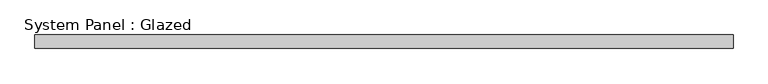
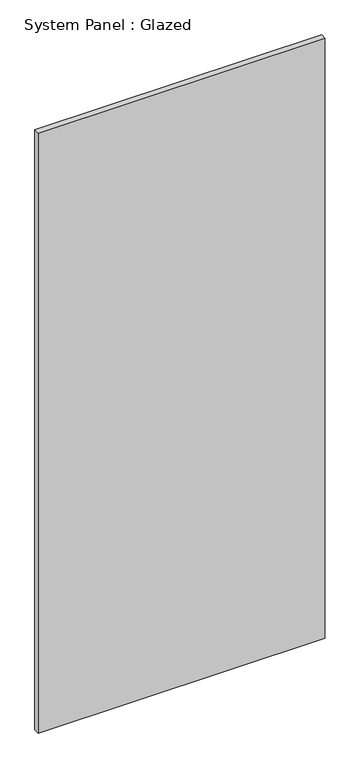
"""IFC4 building model written with IfcOpenShell, lengths in millimetres: plate geometry, System Panel : Glazed."""

from ifc_helpers import new_model, si_unit, origin, origin_with_axes, place, context, project, spatial, polyline, outline, extrude, source, transform, mapped, element, save


def system_panel_glazed_93f0cbb4(model_context):
    return source(origin(), model_context, "Body", "SweptSolid", [
        extrude(outline(polyline([(659.9658525, 19.05), (-659.9658525, 19.05), (-659.9658525, 44.45), (659.9658525, 44.45), (659.9658525, 19.05)])), origin_with_axes(), (0.0, 0.0, 1.0), 2921.0),
    ])


if __name__ == "__main__":
    model = new_model("IFC4")
    model_context = context("Model", 3, world=origin())
    ifc_project = project(units=[si_unit("LENGTHUNIT", "METRE", prefix="MILLI")], contexts=[model_context])
    site = spatial("IfcSite", under=ifc_project)
    building = spatial("IfcBuilding", under=site)
    placement = place(None, origin())
    system_panel_glazed_shape = system_panel_glazed_93f0cbb4(model_context)
    element("IfcPlate", 1, ObjectType="System Panel : Glazed", at=placement, inside=building, context=model_context, shape_type="MappedRepresentation", body=[
        mapped(system_panel_glazed_shape, transform((0.0, 0.0, 0.0), x_axis=(1.0, 0.0, 0.0), y_axis=(0.0, 1.0, 0.0), z_axis=(0.0, 0.0, 1.0))),
    ])
    save(model, "model.ifc")

# Revit data of these elements
# Type "System Panel : Glazed"
#   Construction Type Id = "GSP4R"
#   Analytic Construction = "1/8 in Pilkington single glazing"
#   Visual Light Transmittance = 0.9
#   Solar Heat Gain Coefficient = 0.86
#   Heat Transfer Coefficient (U) = 1.18115 BTU/(h·ft²·°F)
# Element 1 (IfcPlate, "System Panel : Glazed")
#   Materials on its faces: "Glass"
# Materials
#   "Glass": class "Glass", colour RGB 0 128 192, transparency 0.75, Description = "Soda Lime Glass", Cost = 0
